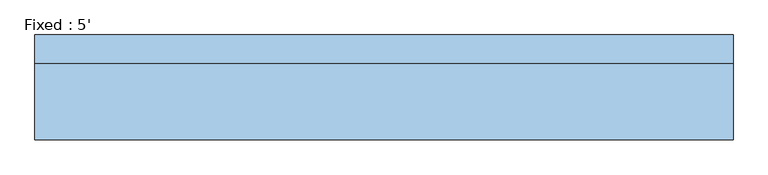
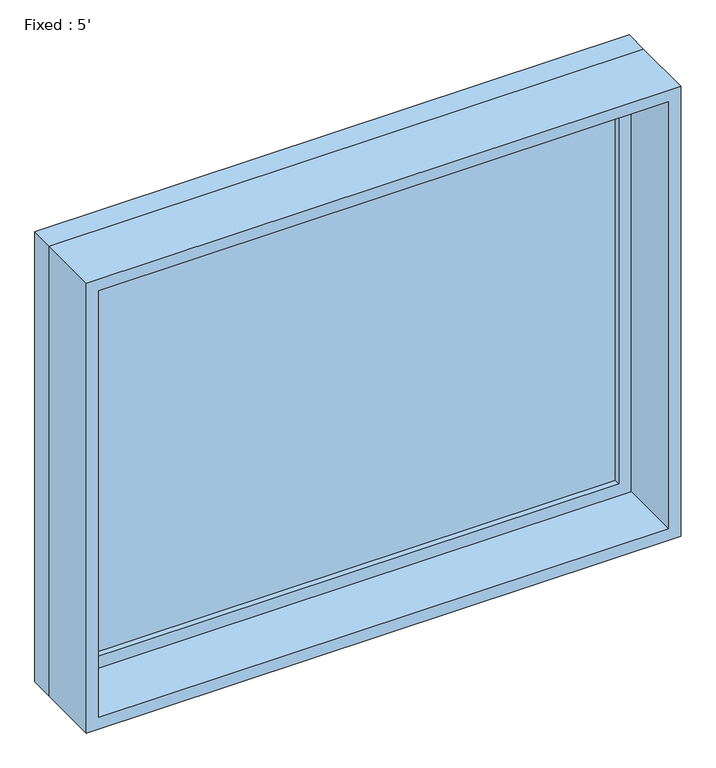
"""IFC4 building model written with IfcOpenShell, lengths in millimetres: window geometry, Fixed : 5'."""

from ifc_helpers import new_model, si_unit, frame, origin, place, context, project, spatial, polyline, outline, extrude, source, transform, mapped, element, save


def fixed_5_145d3b12(model_context):
    return source(origin(), model_context, "Body", "SweptSolid", [
        extrude(outline(polyline([(660.4, 66.675), (-736.6, 66.675), (-736.6, 79.375), (660.4, 79.375), (660.4, 66.675)])), frame((0.0, 0.0, 977.9), z_axis=(0.0, 0.0, 1.0), x_axis=(1.0, 0.0, 0.0)), (0.0, 0.0, 1.0), 1092.2),
        extrude(outline(polyline([(2114.55, -781.05), (933.45, -781.05), (933.45, 704.85), (2114.55, 704.85), (2114.55, -781.05)]), holes=[polyline([(2070.1, -736.6), (2070.1, 660.4), (977.9, 660.4), (977.9, -736.6), (2070.1, -736.6)])]), frame((0.0, 50.8, 0.0), z_axis=(0.0, 1.0, 0.0), x_axis=(0.0, 0.0, 1.0)), (0.0, 0.0, 1.0), 44.45),
        extrude(outline(polyline([(2133.6, -800.1), (914.4, -800.1), (914.4, 723.9), (2133.6, 723.9), (2133.6, -800.1)]), holes=[polyline([(2101.85, -768.35), (2101.85, 692.15), (946.15, 692.15), (946.15, -768.35), (2101.85, -768.35)])]), frame((0.0, -114.3, 0.0), z_axis=(0.0, 1.0, 0.0), x_axis=(0.0, 0.0, 1.0)), (0.0, 0.0, 1.0), 165.1),
        extrude(outline(polyline([(2133.6, 723.9), (2133.6, -800.1), (914.4, -800.1), (914.4, 723.9), (2133.6, 723.9)]), holes=[polyline([(2114.55, 704.85), (933.45, 704.85), (933.45, -781.05), (2114.55, -781.05), (2114.55, 704.85)])]), frame((0.0, 50.8, 0.0), z_axis=(0.0, 1.0, 0.0), x_axis=(0.0, 0.0, 1.0)), (0.0, 0.0, 1.0), 63.5),
    ])


if __name__ == "__main__":
    model = new_model("IFC4")
    model_context = context("Model", 3, world=origin())
    ifc_project = project(units=[si_unit("LENGTHUNIT", "METRE", prefix="MILLI")], contexts=[model_context])
    site = spatial("IfcSite", under=ifc_project)
    building = spatial("IfcBuilding", under=site)
    placement = place(None, origin())
    fixed_5_shape = fixed_5_145d3b12(model_context)
    element("IfcWindow", 1, ObjectType="Fixed : 5'", at=placement, inside=building, context=model_context, shape_type="MappedRepresentation", body=[
        mapped(fixed_5_shape, transform((0.0, 0.0, 0.0), x_axis=(1.0, 0.0, 0.0), y_axis=(0.0, 1.0, 0.0), z_axis=(0.0, 0.0, 1.0))),
    ])
    save(model, "model.ifc")

# Revit data of these elements
# Type "Fixed : 5'"
#   Type Mark = "18"
#   Construction Type Id = "GSP4R"
#   Assembly Code = "B2020100"
#   Analytic Construction = "1/8 in Pilkington single glazing"
#   Visual Light Transmittance = 0.9
#   Solar Heat Gain Coefficient = 0.78
#   Heat Transfer Coefficient (U) = 0.6496 BTU/(h·ft²·°F)
#   Height = 4' - 0"
#   Default Sill Height = 3' - 0"
#   Width = 5' - 0"
#   Window Inset = 0' - 0 3/4"
#   Define Thermal Properties by = 1
#   Glass Pane Material = Glass
#   Sash Material = Sash
#   Wall Closure = (empty or 0)
# Element 1 (IfcWindow, "Fixed : 5'")
#   Materials on its faces: "Sash", "Glass"
# Materials
#   "Glass": class "Glass", colour RGB 0 128 192, transparency 0.75, Description = "Soda Lime Glass", Cost = 0
#   "Sash": class "Wood", colour RGB 224 178 126, transparency 0, Cost = 0
